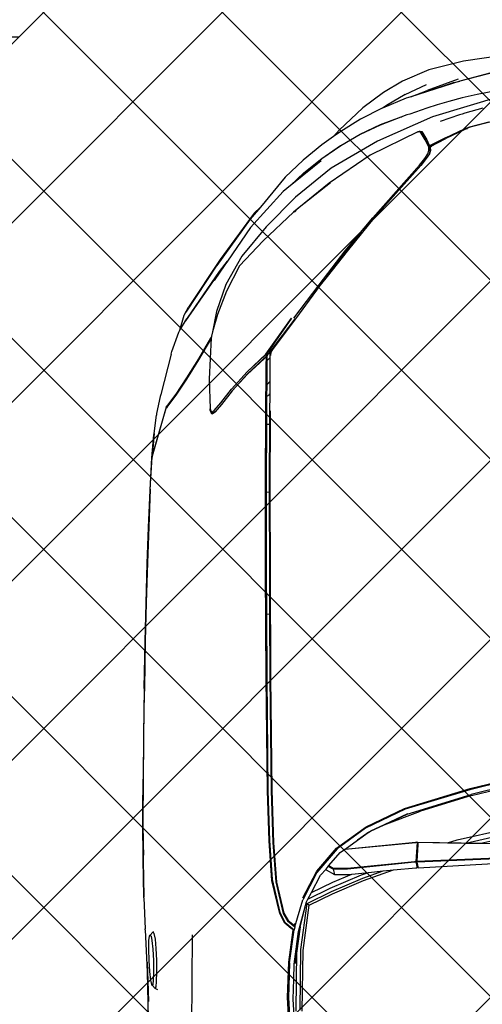
# Model space of a CAD drawing. Units: inches. Extents: x 2167 to 2589, y 1680 to 2489.
# Tile 20 of 38: x 2251 to 2269, y 1796 to 1835. Entities that reach past the tile are written whole.
import ezdxf

# ---------------------------------------------------------------- set-up
doc = ezdxf.new("R2010")
doc.units = ezdxf.units.IN
doc.header["$MEASUREMENT"] = 0
doc.layers.get('0').update_dxf_attribs({"color": 250})
for name, color, linetype, lineweight in [('A-ANNO-DIMS', 2, 'Continuous', 18), ('C-PRKG-VEHS', 8, 'Continuous', 13), ('L-PVMT-PATT', 252, 'Continuous', 13)]:
    doc.layers.add(name, color=color, linetype=linetype, lineweight=lineweight)
doc.layers.add('Edges', color=250, linetype='Continuous')
doc.styles.get("Standard").update_dxf_attribs({"font": 'arial.ttf'})
doc.dimstyles.get("Standard").update_dxf_attribs({"dimtxt": 7, "dimasz": 0.18, "dimexe": 0.18, "dimexo": 0.0625, "dimgap": 0.09, "dimtad": 0, "dimtih": 1, "dimtoh": 1, "dimdec": 1, "dimzin": 0, "dimdsep": 46, "dimlunit": 3, "dimtxsty": 'Standard', "dimcen": 0.09, "dimadec": 0, "dimazin": 0, "dimtfac": 1, "dimtdec": 1, "dimtofl": 0, "dimtmove": 0, "dimatfit": 3, "dimfxl": 1, "dimtolj": 1, "dimtzin": 0, "dimarcsym": 0})

# ---------------------------------------------------------------- blocks, each defined once
blk = doc.blocks.new('Nissan Qashqai pl')
at = {"layer": 'Edges'}
for p, q in [((8.4086, 11.6764), (8.4045, 11.4011)), ((8.4305, 11.3996), (8.419, 11.6758)), ((8.4204, 11.6758), (8.4319, 11.3996)), ((8.4394, 11.4014), (8.4238, 11.6766)), ((7.3497, 11.5674), (7.3653, 11.4838)), ((8.3296, 11.4739), (8.3076, 11.5631)), ((8.3089, 11.5631), (8.3311, 11.4733)), ((8.3157, 11.5647), (8.3377, 11.4753)), ((8.3392, 11.4758), (8.3166, 11.5675)), ((7.3059, 11.5532), (7.3193, 11.4645)), ((8.4009, 11.4559), (8.3792, 11.5515)), ((8.4051, 11.4678), (8.3864, 11.5497)), ((8.4054, 11.4887), (8.3913, 11.5506)), ((7.3297, 11.5237), (7.3467, 11.4596)), ((7.33, 11.5249), (7.3467, 11.4596)), ((7.3676, 11.5172), (7.3963, 11.4215)), ((8.4054, 11.4887), (8.4056, 11.5028)), ((7.3844, 11.4916), (7.3914, 11.4667)), ((7.4101, 11.4733), (7.4033, 11.5005)), ((7.404, 11.5012), (7.4108, 11.4738)), ((8.4051, 11.4678), (8.4054, 11.4887)), ((7.3653, 11.4838), (7.3699, 11.4629)), ((8.3648, 11.3863), (8.3377, 11.4753)), ((8.3392, 11.4758), (8.3608, 11.4048)), ((7.3193, 11.4645), (7.3309, 11.4166)), ((7.3699, 11.4629), (7.375, 11.4442)), ((7.3914, 11.4667), (7.3925, 11.4629)), ((7.3925, 11.4629), (7.3937, 11.4591)), ((7.4115, 11.4695), (7.4101, 11.4733)), ((7.4108, 11.4738), (7.4122, 11.47)), ((7.4131, 11.4659), (7.4115, 11.4695)), ((7.4122, 11.47), (7.4139, 11.4664)), ((7.4126, 11.47), (7.4125, 11.4702)), ((7.4132, 11.4685), (7.4126, 11.47)), ((7.4255, 11.4398), (7.4131, 11.4659)), ((7.4139, 11.4664), (7.4267, 11.4401)), ((8.3573, 11.3824), (8.3296, 11.4739)), ((8.3311, 11.4733), (8.3582, 11.3836)), ((8.4048, 11.4423), (8.4051, 11.4678)), ((7.344, 11.4572), (7.3596, 11.4139)), ((7.3489, 11.4517), (7.3467, 11.4596)), ((7.3467, 11.4596), (7.3686, 11.3913)), ((7.3489, 11.4517), (7.3686, 11.3913)), ((7.3937, 11.4591), (7.4029, 11.4321)), ((8.4048, 11.4423), (8.4009, 11.4559)), ((7.375, 11.4442), (7.3799, 11.4278)), ((7.4255, 11.4398), (7.4367, 11.4174)), ((7.4379, 11.4179), (7.4267, 11.4401)), ((8.4041, 11.4013), (8.4048, 11.4423)), ((7.3799, 11.4278), (7.3845, 11.4136)), ((7.3963, 11.4215), (7.4302, 11.3449)), ((7.4375, 11.42), (7.4384, 11.4182)), ((7.3309, 11.4166), (7.347, 11.3798)), ((7.3655, 11.3837), (7.3514, 11.4133)), ((7.3686, 11.3913), (7.3596, 11.4139)), ((7.3845, 11.4136), (7.3925, 11.3899)), ((7.4167, 11.4049), (7.417, 11.4065)), ((7.4282, 11.4113), (7.4169, 11.4044)), ((7.417, 11.4065), (7.4283, 11.4135)), ((7.4296, 11.4129), (7.4183, 11.406)), ((7.4387, 11.4162), (7.4282, 11.4113)), ((7.4283, 11.4135), (7.4359, 11.417)), ((7.4296, 11.4129), (7.4383, 11.417)), ((7.4359, 11.417), (7.4367, 11.4174)), ((7.4383, 11.417), (7.4367, 11.4174)), ((7.4379, 11.4179), (7.4384, 11.4182)), ((7.4389, 11.4173), (7.4379, 11.4179)), ((7.4383, 11.417), (7.4379, 11.4179)), ((7.4389, 11.4173), (7.4383, 11.417)), ((7.4384, 11.4182), (7.4387, 11.4183)), ((7.4387, 11.4183), (7.443, 11.4188)), ((7.4431, 11.4166), (7.4387, 11.4162)), ((7.4389, 11.4173), (7.44, 11.4178)), ((7.4442, 11.4183), (7.44, 11.4178)), ((7.443, 11.4188), (7.4477, 11.4172)), ((7.4479, 11.4149), (7.4431, 11.4166)), ((7.4477, 11.4172), (7.4442, 11.4183)), ((7.4477, 11.4172), (7.4541, 11.4128)), ((7.4541, 11.4108), (7.4479, 11.4149)), ((7.4541, 11.4128), (7.4638, 11.4051)), ((7.4635, 11.4034), (7.4541, 11.4108)), ((7.4172, 11.4047), (7.4167, 11.4049)), ((7.4169, 11.4036), (7.4167, 11.4049)), ((7.4172, 11.4047), (7.4169, 11.4044)), ((7.4169, 11.4044), (7.4169, 11.4036)), ((7.4172, 11.4018), (7.4169, 11.4036)), ((7.4169, 11.4036), (7.4169, 11.403)), ((7.4169, 11.403), (7.4172, 11.4011)), ((7.4183, 11.406), (7.4172, 11.4047)), ((7.4174, 11.4013), (7.4172, 11.4018)), ((7.4172, 11.4011), (7.4498, 11.3349)), ((7.4174, 11.4013), (7.4175, 11.4012)), ((7.5369, 11.3385), (7.4635, 11.4034)), ((7.4638, 11.4051), (7.5371, 11.34)), ((8.3799, 11.3545), (8.3608, 11.4048)), ((8.407, 11.401), (8.4037, 11.4002)), ((8.4037, 11.4002), (8.4314, 11.3985)), ((8.4037, 11.3992), (8.4037, 11.4002)), ((8.4037, 11.3992), (8.4046, 11.3981)), ((8.4042, 11.3983), (8.4037, 11.3992)), ((8.4041, 11.4013), (8.4045, 11.4011)), ((8.4134, 11.3049), (8.4042, 11.3983)), ((8.4045, 11.4011), (8.407, 11.401)), ((8.4046, 11.3981), (8.4138, 11.3048)), ((8.407, 11.401), (8.4305, 11.3996)), ((8.4305, 11.3996), (8.4319, 11.3996)), ((8.4306, 11.3966), (8.4314, 11.3975)), ((8.4398, 11.3032), (8.4306, 11.3966)), ((8.4314, 11.3985), (8.4394, 11.4004)), ((8.4314, 11.3985), (8.4314, 11.3975)), ((8.4314, 11.3975), (8.4319, 11.3967)), ((8.4319, 11.3996), (8.436, 11.4006)), ((8.4319, 11.3967), (8.4412, 11.3033)), ((8.436, 11.4006), (8.4394, 11.4014)), ((8.4394, 11.4004), (8.436, 11.4006)), ((8.4394, 11.3984), (8.4394, 11.4004)), ((8.4425, 11.3672), (8.4394, 11.3984)), ((7.347, 11.3798), (7.3624, 11.3535)), ((7.3655, 11.3837), (7.3805, 11.3576)), ((7.3686, 11.3913), (7.3707, 11.3849)), ((7.3707, 11.3849), (7.3843, 11.3522)), ((7.3925, 11.3899), (7.3938, 11.3859)), ((7.3938, 11.3859), (7.3951, 11.3822)), ((7.3951, 11.3822), (7.3965, 11.3787)), ((8.3826, 11.3291), (8.3573, 11.3824)), ((8.3582, 11.3836), (8.3844, 11.3284)), ((8.3646, 11.387), (8.3799, 11.3545)), ((8.3888, 11.3355), (8.3648, 11.3863)), ((7.3962, 11.3781), (7.3965, 11.3787)), ((7.4071, 11.3493), (7.3962, 11.3781)), ((7.3965, 11.3787), (7.3969, 11.3777)), ((7.3969, 11.3777), (7.4078, 11.349)), ((8.4571, 11.3258), (8.4425, 11.3672)), ((8.4439, 11.3531), (8.4425, 11.3672)), ((7.3624, 11.3535), (7.3837, 11.3245)), ((7.3805, 11.3576), (7.3843, 11.3522)), ((7.3843, 11.3522), (7.3845, 11.3517)), ((7.3845, 11.3517), (7.3997, 11.3215)), ((8.3799, 11.3545), (8.3888, 11.3355)), ((8.454, 11.3245), (8.4439, 11.3531)), ((8.4459, 11.3326), (8.4439, 11.3531)), ((7.4205, 11.3212), (7.4071, 11.3493)), ((7.4078, 11.349), (7.4211, 11.321)), ((7.4302, 11.3449), (7.4679, 11.2807)), ((7.5827, 11.3001), (7.5369, 11.3385)), ((7.5371, 11.34), (7.5568, 11.324)), ((7.3837, 11.3245), (7.4147, 11.2918)), ((7.4498, 11.3349), (7.4884, 11.2778)), ((8.4122, 11.2883), (8.3826, 11.3291)), ((8.3844, 11.3284), (8.4134, 11.2888)), ((8.3901, 11.3328), (8.3888, 11.3355)), ((8.3901, 11.3328), (8.4011, 11.3173)), ((8.3904, 11.3321), (8.3901, 11.3328)), ((8.4011, 11.3173), (8.3904, 11.3321)), ((8.4493, 11.3229), (8.4459, 11.3326)), ((8.4482, 11.3095), (8.4459, 11.3326)), ((8.4725, 11.2812), (8.454, 11.3245)), ((8.4756, 11.2826), (8.4571, 11.3258)), ((7.3997, 11.3215), (7.4166, 11.2939)), ((7.4363, 11.294), (7.4205, 11.3212)), ((7.4211, 11.321), (7.4369, 11.2938)), ((7.584, 11.3013), (7.5568, 11.324)), ((7.5568, 11.324), (7.5829, 11.303)), ((8.4135, 11.3), (8.4011, 11.3173)), ((8.468, 11.2793), (8.4493, 11.3229)), ((7.6296, 11.2639), (7.5827, 11.3001)), ((7.5829, 11.303), (7.618, 11.275)), ((7.618, 11.275), (7.584, 11.3013)), ((8.4135, 11.3), (8.4134, 11.3049)), ((8.4139, 11.2994), (8.4135, 11.3)), ((8.4138, 11.3048), (8.4139, 11.2994)), ((8.4183, 11.2934), (8.4139, 11.2994)), ((8.44, 11.2834), (8.4398, 11.3032)), ((8.4412, 11.3033), (8.4415, 11.2835)), ((8.4594, 11.2831), (8.4482, 11.3095)), ((8.4487, 11.305), (8.4482, 11.3095)), ((8.4489, 11.2852), (8.4487, 11.305)), ((7.4147, 11.2918), (7.4239, 11.2837)), ((7.4166, 11.2939), (7.4239, 11.2837)), ((7.4239, 11.2837), (7.4354, 11.2675)), ((7.4542, 11.2677), (7.4363, 11.294)), ((7.4369, 11.2938), (7.4549, 11.2675)), ((8.4444, 11.2608), (8.4122, 11.2883)), ((8.4134, 11.2888), (8.4462, 11.2609)), ((8.4365, 11.2776), (8.4183, 11.2934)), ((8.4365, 11.2776), (8.44, 11.2834)), ((8.4415, 11.2835), (8.4375, 11.2767)), ((8.4415, 11.2835), (8.4489, 11.2852)), ((8.4422, 11.2737), (8.4489, 11.2852)), ((7.4679, 11.2807), (7.5081, 11.2311)), ((7.4882, 11.2797), (7.5243, 11.2341)), ((7.4884, 11.2778), (7.5289, 11.2283)), ((7.618, 11.275), (7.6301, 11.2654)), ((8.4375, 11.2767), (8.4365, 11.2776)), ((8.4412, 11.2735), (8.4375, 11.2767)), ((8.4422, 11.2737), (8.4412, 11.2735)), ((8.4499, 11.2659), (8.4412, 11.2735)), ((8.4737, 11.2534), (8.4594, 11.2831)), ((8.4831, 11.2484), (8.468, 11.2793)), ((8.4889, 11.2473), (8.4725, 11.2812)), ((8.4914, 11.25), (8.4756, 11.2826)), ((7.4354, 11.2675), (7.4565, 11.2419)), ((7.4744, 11.2427), (7.4542, 11.2677)), ((7.4549, 11.2675), (7.475, 11.2426)), ((7.4574, 11.267), (7.4885, 11.2283)), ((7.676, 11.2289), (7.6296, 11.2639)), ((7.6301, 11.2654), (7.6306, 11.2651)), ((7.6306, 11.2651), (7.6306, 11.265)), ((7.6306, 11.265), (7.6373, 11.2601)), ((7.6373, 11.2601), (7.6769, 11.2312)), ((8.4814, 11.2413), (8.4444, 11.2608)), ((8.4462, 11.2609), (8.4838, 11.2415)), ((8.4737, 11.2534), (8.4499, 11.2659)), ((7.4918, 11.2242), (7.4744, 11.2427)), ((7.475, 11.2426), (7.477, 11.2404)), ((8.4831, 11.2484), (8.4737, 11.2534)), ((8.4867, 11.2465), (8.4831, 11.2484)), ((8.528, 11.2354), (8.4867, 11.2465)), ((8.5214, 11.2374), (8.4867, 11.2465)), ((8.4889, 11.2473), (8.4914, 11.25)), ((8.5531, 11.2387), (8.4889, 11.2473)), ((8.5544, 11.2416), (8.4914, 11.25)), ((7.4565, 11.2419), (7.4801, 11.2168)), ((7.477, 11.2404), (7.4765, 11.2411)), ((7.477, 11.2405), (7.4775, 11.2399)), ((7.4784, 11.2388), (7.477, 11.2404)), ((7.477, 11.2404), (7.4775, 11.2399)), ((7.4775, 11.2399), (7.4787, 11.2385)), ((7.4775, 11.2399), (7.4787, 11.2387)), ((7.4787, 11.2387), (7.4782, 11.2392)), ((7.4795, 11.2377), (7.4787, 11.2387)), ((7.4787, 11.2387), (7.4885, 11.2283)), ((7.5081, 11.2311), (7.5492, 11.1902)), ((7.5243, 11.2341), (7.5286, 11.2296)), ((7.6769, 11.2312), (7.7194, 11.1992)), ((7.7232, 11.1955), (7.6771, 11.2307)), ((8.5216, 11.2303), (8.4838, 11.2415)), ((8.5132, 11.2202), (8.5216, 11.2303)), ((8.5155, 11.2168), (8.5258, 11.2291)), ((8.5197, 11.2297), (8.5166, 11.2307)), ((8.5177, 11.2272), (8.5197, 11.2297)), ((8.5216, 11.2303), (8.5197, 11.2297)), ((8.5214, 11.2374), (8.555, 11.233)), ((8.5301, 11.2352), (8.5214, 11.2374)), ((8.5216, 11.2303), (8.5258, 11.2291)), ((8.5258, 11.2291), (8.5259, 11.2279)), ((8.5715, 11.2227), (8.5258, 11.2291)), ((8.5736, 11.2291), (8.528, 11.2354)), ((8.6375, 11.2376), (8.5531, 11.2387)), ((8.6386, 11.2404), (8.5544, 11.2416)), ((8.6387, 11.2319), (8.555, 11.233)), ((8.555, 11.233), (8.5726, 11.2307)), ((8.5941, 11.2286), (8.5736, 11.2291)), ((8.5941, 11.2289), (8.5941, 11.2286)), ((8.622, 11.228), (8.5941, 11.2286)), ((8.6699, 11.231), (8.622, 11.228)), ((7.4801, 11.2168), (7.5217, 11.1823)), ((7.4885, 11.2283), (7.4918, 11.2242)), ((7.4918, 11.2242), (7.5001, 11.2139)), ((7.5289, 11.2283), (7.5687, 11.1862)), ((7.7261, 11.1898), (7.6762, 11.2256)), ((7.6762, 11.2256), (7.7233, 11.1928)), ((8.5155, 11.2168), (8.5018, 11.2098)), ((8.5025, 11.2148), (8.5125, 11.221)), ((8.5163, 11.2162), (8.5029, 11.2092)), ((8.5032, 11.2141), (8.5132, 11.2202)), ((8.5125, 11.221), (8.5177, 11.2272)), ((8.5237, 11.2252), (8.5163, 11.2162)), ((8.5259, 11.2279), (8.5237, 11.2252)), ((8.5294, 11.2274), (8.5259, 11.2279)), ((8.5706, 11.2216), (8.5294, 11.2274)), ((8.6197, 11.2201), (8.5706, 11.2216)), ((8.5715, 11.2227), (8.6203, 11.2213)), ((8.6683, 11.2226), (8.6197, 11.2201)), ((8.6203, 11.2213), (8.6721, 11.2241)), ((7.5001, 11.2139), (7.5501, 11.1684)), ((8.4042, 11.1995), (8.4588, 11.2036)), ((8.4049, 11.2004), (8.4595, 11.2047)), ((8.5018, 11.2098), (8.4559, 11.1991)), ((8.5029, 11.2092), (8.4571, 11.1983)), ((8.4588, 11.2036), (8.5032, 11.2141)), ((8.4595, 11.2047), (8.5025, 11.2148)), ((7.5492, 11.1902), (7.59, 11.1565)), ((7.7194, 11.1992), (7.7232, 11.1966)), ((7.7232, 11.1966), (7.7279, 11.1965)), ((7.7281, 11.1918), (7.7232, 11.1955)), ((7.7232, 11.1955), (7.7245, 11.1955)), ((7.7267, 11.1902), (7.7233, 11.1928)), ((7.7247, 11.1954), (7.7245, 11.1955)), ((7.7245, 11.1955), (7.7294, 11.1955)), ((7.7261, 11.1898), (7.7507, 11.1638)), ((7.7286, 11.1881), (7.7267, 11.1902)), ((7.7281, 11.1918), (7.7299, 11.1904)), ((7.7349, 11.1917), (7.7281, 11.1918)), ((7.753, 11.1648), (7.7281, 11.1918)), ((7.7507, 11.1638), (7.7286, 11.1881)), ((7.7294, 11.1955), (7.731, 11.1955)), ((7.7299, 11.1904), (7.7324, 11.1876)), ((7.7299, 11.1904), (7.7364, 11.1904)), ((7.731, 11.1955), (7.7349, 11.1917)), ((7.731, 11.1955), (7.764, 11.1953)), ((7.7324, 11.1876), (7.7539, 11.1642)), ((7.768, 11.1915), (7.7349, 11.1917)), ((7.7363, 11.1904), (7.7364, 11.1904)), ((7.7694, 11.1901), (7.7364, 11.1904)), ((7.764, 11.1953), (7.7636, 11.1957)), ((7.768, 11.1915), (7.764, 11.1953)), ((7.764, 11.1953), (7.7662, 11.1953)), ((7.7659, 11.1957), (7.7662, 11.1953)), ((7.7662, 11.1953), (7.7668, 11.1946)), ((7.7662, 11.1953), (7.7811, 11.1952)), ((7.7692, 11.1915), (7.768, 11.1915)), ((7.7694, 11.1901), (7.7687, 11.1908)), ((7.7844, 11.1913), (7.7692, 11.1915)), ((7.7707, 11.1901), (7.7694, 11.1901)), ((7.7851, 11.19), (7.7707, 11.1901)), ((7.7811, 11.1952), (7.7809, 11.1958)), ((7.7814, 11.1946), (7.7811, 11.1952)), ((7.7811, 11.1952), (7.7822, 11.1952)), ((7.7822, 11.1952), (7.7819, 11.1958)), ((7.7822, 11.1952), (7.8057, 11.195)), ((7.7844, 11.1913), (7.7822, 11.1952)), ((7.8078, 11.1911), (7.7844, 11.1913)), ((7.7846, 11.1909), (7.7851, 11.19)), ((7.8083, 11.1898), (7.7851, 11.19)), ((7.8048, 11.1959), (7.8233, 11.1958)), ((7.8057, 11.195), (7.8233, 11.195)), ((7.8233, 11.1911), (7.8078, 11.1911)), ((7.904, 11.1894), (7.8083, 11.1898)), ((7.8233, 11.195), (7.8233, 11.1958)), ((7.8233, 11.1958), (7.9014, 11.1955)), ((7.8233, 11.195), (7.902, 11.1947)), ((7.8233, 11.1911), (7.8233, 11.195)), ((7.8233, 11.1899), (7.8233, 11.1911)), ((7.9036, 11.1907), (7.8233, 11.1911)), ((7.9014, 11.1955), (7.9185, 11.1955)), ((7.902, 11.1947), (7.9183, 11.1947)), ((7.9176, 11.1908), (7.9036, 11.1907)), ((8.0276, 11.1896), (7.904, 11.1894)), ((7.9183, 11.1947), (7.9176, 11.1908)), ((8.0275, 11.1909), (7.9176, 11.1908)), ((7.9185, 11.1955), (7.9183, 11.1947)), ((7.9183, 11.1947), (8.0275, 11.1948)), ((7.9185, 11.1955), (8.0273, 11.1957)), ((8.0273, 11.1957), (8.1753, 11.1963)), ((8.0275, 11.1948), (8.0876, 11.1951)), ((8.0873, 11.1911), (8.0275, 11.1909)), ((8.1753, 11.1903), (8.0276, 11.1896)), ((8.0876, 11.1951), (8.0873, 11.1911)), ((8.1755, 11.1915), (8.0873, 11.1911)), ((8.0876, 11.1951), (8.1754, 11.1954)), ((8.1753, 11.1963), (8.3318, 11.198)), ((8.3324, 11.192), (8.1753, 11.1903)), ((8.1754, 11.1954), (8.332, 11.1971)), ((8.3324, 11.1931), (8.1755, 11.1915)), ((8.3318, 11.198), (8.4049, 11.2004)), ((8.332, 11.1971), (8.4042, 11.1995)), ((8.4014, 11.1953), (8.3324, 11.1931)), ((8.4022, 11.1943), (8.3324, 11.192)), ((8.4559, 11.1991), (8.4014, 11.1953)), ((8.4571, 11.1983), (8.4022, 11.1943)), ((7.5304, 11.1737), (7.5217, 11.1823)), ((7.5217, 11.1823), (7.5387, 11.1682)), ((7.5687, 11.1862), (7.6032, 11.1533)), ((7.5304, 11.1737), (7.5946, 11.1262)), ((7.5387, 11.1682), (7.6031, 11.1217)), ((7.5501, 11.1684), (7.5969, 11.1365)), ((7.7748, 11.1423), (7.7507, 11.1638)), ((7.753, 11.1648), (7.7772, 11.1431)), ((7.7539, 11.1642), (7.7772, 11.1431)), ((7.59, 11.1565), (7.6295, 11.1344)), ((7.6032, 11.1533), (7.6386, 11.1353)), ((7.6113, 11.1256), (7.5969, 11.1365)), ((7.5969, 11.1365), (7.6021, 11.1329)), ((7.6021, 11.1329), (7.6118, 11.1255)), ((7.6021, 11.1329), (7.6237, 11.1181)), ((7.6295, 11.1344), (7.667, 11.1212)), ((7.6386, 11.1353), (7.6708, 11.1225)), ((7.7938, 11.1271), (7.7748, 11.1423)), ((7.7772, 11.1431), (7.7959, 11.1281)), ((7.5946, 11.1262), (7.6608, 11.0825)), ((7.6676, 11.0791), (7.6024, 11.1221)), ((7.6759, 11.0809), (7.6113, 11.1256)), ((7.6118, 11.1255), (7.6799, 11.0783)), ((7.667, 11.1212), (7.6949, 11.1158)), ((7.6708, 11.1225), (7.6949, 11.1158)), ((7.8045, 11.1179), (7.7938, 11.1271)), ((7.7959, 11.1281), (7.8062, 11.1192)), ((7.8087, 11.1159), (7.8062, 11.1192)), ((7.8062, 11.1192), (7.8066, 11.1188)), ((7.6949, 11.1158), (7.701, 11.1141)), ((7.701, 11.1141), (7.7024, 11.1141)), ((7.7038, 11.1132), (7.7024, 11.1141)), ((7.7024, 11.1141), (7.7034, 11.114)), ((7.7034, 11.114), (7.7056, 11.1128)), ((7.7034, 11.114), (7.7608, 11.1112)), ((7.7325, 11.0966), (7.7038, 11.1132)), ((7.7056, 11.1128), (7.7341, 11.0963)), ((7.7608, 11.1112), (7.8014, 11.1124)), ((7.8014, 11.1124), (7.8022, 11.1126)), ((7.8022, 11.1126), (7.8072, 11.1141)), ((7.8037, 11.1126), (7.8022, 11.1126)), ((7.8096, 11.1148), (7.8037, 11.1126)), ((7.8072, 11.1141), (7.8045, 11.1179)), ((7.8066, 11.1188), (7.8096, 11.1148)), ((7.8072, 11.1141), (7.8087, 11.1159)), ((7.7591, 11.08), (7.7325, 11.0966)), ((7.7341, 11.0963), (7.7606, 11.0798)), ((7.6712, 11.0767), (7.6608, 11.0825)), ((7.6793, 11.0784), (7.6759, 11.0809)), ((7.6802, 11.0782), (7.6793, 11.0784)), ((7.6802, 11.0782), (7.6799, 11.0783)), ((7.6809, 11.0777), (7.6802, 11.0782)), ((7.7814, 11.065), (7.7591, 11.08)), ((7.7606, 11.0798), (7.7828, 11.0649)), ((8.5326, 11.0874), (8.6675, 11.0866)), ((7.6721, 11.0762), (7.6712, 11.0767)), ((7.6926, 11.0705), (7.6721, 11.0762)), ((7.6926, 11.0705), (7.6809, 11.0777)), ((7.6953, 11.0688), (7.6926, 11.0705)), ((7.7223, 11.059), (7.6953, 11.0688)), ((7.797, 11.0534), (7.7814, 11.065)), ((7.7828, 11.0649), (7.7984, 11.0533)), ((7.7262, 11.0581), (7.7223, 11.059)), ((7.7262, 11.0581), (7.7819, 11.0438)), ((7.797, 11.0534), (7.797, 11.0534)), ((7.7998, 11.0513), (7.797, 11.0534)), ((7.7984, 11.0533), (7.8007, 11.0516)), ((7.7998, 11.0513), (7.8676, 11.0318)), ((7.8007, 11.0516), (7.8002, 11.0517)), ((7.8007, 11.0516), (7.8012, 11.0513)), ((7.8681, 11.032), (7.8012, 11.0513)), ((7.7819, 11.0438), (7.7848, 11.043)), ((7.7848, 11.043), (7.8087, 11.038)), ((7.8087, 11.038), (7.8106, 11.0377)), ((7.8107, 11.0377), (7.8106, 11.0377)), ((7.8363, 11.0344), (7.8107, 11.0377)), ((8.5518, 11.0375), (8.5385, 11.0363)), ((8.568, 11.0382), (8.5518, 11.0375)), ((8.5842, 11.0384), (8.568, 11.0382)), ((8.5974, 11.0381), (8.5842, 11.0384)), ((8.6049, 11.0373), (8.5974, 11.0381)), ((8.6073, 11.0362), (8.6049, 11.0373)), ((8.609, 11.0397), (8.6073, 11.0362)), ((7.8381, 11.0342), (7.8363, 11.0344)), ((7.8363, 11.0344), (7.8676, 11.0318)), ((7.87, 11.0315), (7.8381, 11.0342)), ((7.8681, 11.032), (7.8676, 11.0318)), ((7.8681, 11.032), (7.869, 11.0317)), ((7.9137, 11.0292), (7.869, 11.0317)), ((7.9151, 11.029), (7.87, 11.0315)), ((7.9137, 11.0292), (7.9658, 11.027)), ((7.9668, 11.0268), (7.9151, 11.029)), ((7.9658, 11.027), (8.016, 11.0253)), ((8.0168, 11.0251), (7.9668, 11.0268)), ((8.016, 11.0253), (8.0713, 11.0237)), ((8.0718, 11.0235), (8.0168, 11.0251)), ((8.0713, 11.0237), (8.1249, 11.0223)), ((8.1251, 11.0222), (8.0718, 11.0235)), ((8.5259, 11.0221), (8.5838, 11.0251)), ((8.5283, 11.0336), (8.5287, 11.0329)), ((8.531, 11.0346), (8.5287, 11.0329)), ((8.5287, 11.0329), (8.5331, 11.0292)), ((8.5385, 11.0363), (8.531, 11.0346)), ((8.5331, 11.0292), (8.5346, 11.0303)), ((8.5347, 11.0282), (8.5331, 11.0292)), ((8.5346, 11.0303), (8.5406, 11.0316)), ((8.5407, 11.0274), (8.5347, 11.0282)), ((8.5406, 11.0316), (8.5526, 11.0328)), ((8.5527, 11.0273), (8.5407, 11.0274)), ((8.5526, 11.0328), (8.5681, 11.0335)), ((8.5682, 11.0278), (8.5527, 11.0273)), ((8.5681, 11.0335), (8.5836, 11.0337)), ((8.5837, 11.0288), (8.5682, 11.0278)), ((8.5707, 11.0248), (8.5965, 11.0258)), ((8.5836, 11.0337), (8.5957, 11.0334)), ((8.5958, 11.0301), (8.5837, 11.0288)), ((8.5838, 11.0251), (8.6489, 11.0263)), ((8.5838, 11.0251), (8.5965, 11.0258)), ((8.5957, 11.0334), (8.6017, 11.0328)), ((8.6018, 11.0312), (8.5958, 11.0301)), ((8.5965, 11.0258), (8.6252, 11.0268)), ((8.6017, 11.0328), (8.6032, 11.0321)), ((8.6032, 11.0321), (8.6018, 11.0312)), ((8.6073, 11.0362), (8.6032, 11.0321)), ((8.1249, 11.0223), (8.1901, 11.021)), ((8.1902, 11.0208), (8.1251, 11.0222)), ((8.1901, 11.021), (8.1938, 11.021)), ((8.1902, 11.021), (8.1938, 11.021)), ((8.1904, 11.0209), (8.1902, 11.0208)), ((8.1904, 11.0209), (8.2543, 11.0198)), ((8.1938, 11.021), (8.1954, 11.0209)), ((8.1954, 11.0209), (8.2544, 11.02)), ((8.2544, 11.0198), (8.2543, 11.0199)), ((8.2543, 11.0198), (8.2544, 11.0198)), ((8.2544, 11.02), (8.3166, 11.0193)), ((8.2544, 11.0198), (8.2556, 11.0198)), ((8.2556, 11.0198), (8.256, 11.0198)), ((8.256, 11.0198), (8.2561, 11.0198)), ((8.2561, 11.0198), (8.2693, 11.0197)), ((8.2693, 11.0197), (8.2694, 11.0197)), ((8.2694, 11.0197), (8.3098, 11.0192)), ((8.3098, 11.0192), (8.3163, 11.0192)), ((8.3663, 11.019), (8.3163, 11.0192)), ((8.3597, 11.019), (8.3163, 11.0192)), ((8.3166, 11.0193), (8.3764, 11.0191)), ((8.3602, 11.019), (8.3597, 11.019)), ((8.3608, 11.019), (8.3602, 11.019)), ((8.3663, 11.019), (8.3608, 11.019)), ((8.3663, 11.019), (8.3764, 11.0191)), ((8.3757, 11.019), (8.3663, 11.019)), ((8.4282, 11.0193), (8.3757, 11.019)), ((8.3764, 11.0191), (8.4069, 11.0192)), ((8.4069, 11.0192), (8.4219, 11.0196)), ((8.4069, 11.0192), (8.4292, 11.0193)), ((8.4799, 11.0202), (8.4282, 11.0193)), ((8.4292, 11.0193), (8.4799, 11.0202)), ((8.4811, 11.0203), (8.4799, 11.0202)), ((8.4811, 11.0203), (8.5241, 11.022)), ((8.5259, 11.0221), (8.5241, 11.022))]:
    blk.add_line(p, q, dxfattribs=at)
blk = doc.blocks.new('car')
blk.add_blockref('Nissan Qashqai pl', (-9.7433, -11.9151))
blk = doc.blocks.new('carr')
blk.add_blockref('car', (0.5124, -0.007))
blk = doc.blocks.new('*D45')
at = {"layer": 'A-ANNO-DIMS', "color": 0, "lineweight": -2, "transparency": 16777216}
for p, q in [((2251.156, 1833.955), (2232.359, 1833.955)), ((2232.539, 1833.775), (2232.539, 1775.399)), ((2232.539, 1709.605), (2232.539, 1767.981)), ((2251.156, 1709.425), (2232.359, 1709.425))]:
    blk.add_line(p, q, dxfattribs=at)
at = {"layer": 'A-ANNO-DIMS', "color": 0, "transparency": 16777216}
for points in [[(2232.509, 1833.775), (2232.569, 1833.775), (2232.539, 1833.955)], [(2232.509, 1709.605), (2232.569, 1709.605), (2232.539, 1709.425)]]:
    blk.add_solid(points, dxfattribs=at)
at = {"layer": 'Defpoints', "color": 0, "transparency": 16777216}
for p in [(2251.218, 1833.955), (2232.539, 1709.425), (2251.218, 1709.425)]:
    blk.add_point(p, dxfattribs=at)
at = {"layer": 'A-ANNO-DIMS', "color": 0, "transparency": 16777216, "insert": (2232.539, 1771.69), "char_height": 7, "attachment_point": 5}
blk.add_mtext('\\A1;CAR 10\'-4 1/2" TYP.', dxfattribs=at)

msp = doc.modelspace()

# ---------------------------------------------------------------- hatches: boundary and pattern name
at = {"layer": 'L-PVMT-PATT'}
h = msp.add_hatch(dxfattribs=at)
h.set_pattern_fill('ANSI37', color=256, scale=40)
h.paths.add_polyline_path([(2417.548, 1783.695), (2417.548, 1846.042), (2239.361, 1846.042), (2239.361, 1687.695), (2369.843, 1687.695), (2369.843, 1696.695), (2375.607, 1696.695), (2416.107, 1696.695), (2417.548, 1696.695)])

# ---------------------------------------------------------------- block references
at = {"layer": 'C-PRKG-VEHS', "xscale": 28.42784210623918, "yscale": 28.42784210623918, "zscale": 28.42784210623918, "rotation": 270}
msp.add_blockref('carr', (2281.736, 1778.659), dxfattribs=at)

# ---------------------------------------------------------------- dimensions: what is measured, and where the dimension line sits
at = {"layer": 'A-ANNO-DIMS'}
dim = msp.add_linear_dim(base=(2232.539, 1709.425), p1=(2251.218, 1833.955), p2=(2251.218, 1709.425), angle=270, text='CAR <> TYP.', dimstyle='Standard', override={"dimdec": 1, "dimlfac": 1, "dimrnd": 0, "dimzin": 1, "dimdsep": 46, "dimlunit": 4, "dimfrac": 2}, dxfattribs=at)
dim.commit()
dim.dimension.update_dxf_attribs({"geometry": '*D45', "text_midpoint": (2232.539, 1771.69)})

doc.saveas('drawing.dxf')
